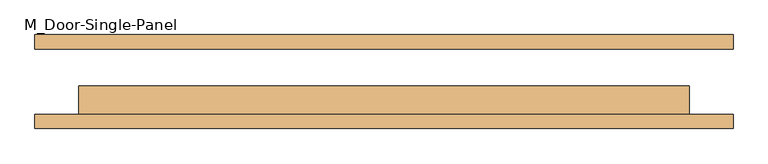
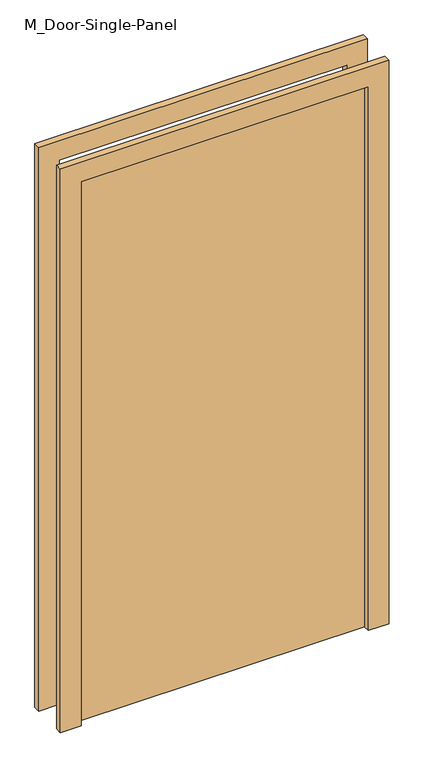
"""IFC4 building model written with IfcOpenShell, lengths in millimetres: door geometry, M_Door-Single-Panel."""

from ifc_helpers import new_model, si_unit, frame, origin, origin_with_axes, place, context, project, spatial, polyline, outline, extrude, source, transform, mapped, element, save


def m_door_single_panel_05506f71(model_context):
    return source(origin(), model_context, "Body", "SweptSolid", [
        extrude(outline(polyline([(533.4, -7.15), (533.4, -57.15), (-533.4, -57.15), (-533.4, -7.15), (533.4, -7.15)])), origin_with_axes(), (0.0, 0.0, 1.0), 2133.6),
        extrude(outline(polyline([(2209.8, 609.6), (2209.8, -609.6), (0.0, -609.6), (0.0, -533.4), (2133.6, -533.4), (2133.6, 533.4), (0.0, 533.4), (0.0, 609.6), (2209.8, 609.6)])), frame((0.0, 57.15, 0.0), z_axis=(0.0, 1.0, 0.0), x_axis=(0.0, 0.0, 1.0)), (0.0, 0.0, 1.0), 25.0),
        extrude(outline(polyline([(2209.8, -609.6), (0.0, -609.6), (0.0, -533.4), (2133.6, -533.4), (2133.6, 533.4), (0.0, 533.4), (0.0, 609.6), (2209.8, 609.6), (2209.8, -609.6)])), frame((0.0, -82.15, 0.0), z_axis=(0.0, 1.0, 0.0), x_axis=(0.0, 0.0, 1.0)), (0.0, 0.0, 1.0), 25.0),
    ])


if __name__ == "__main__":
    model = new_model("IFC4")
    model_context = context("Model", 3, world=origin())
    ifc_project = project(units=[si_unit("LENGTHUNIT", "METRE", prefix="MILLI")], contexts=[model_context])
    site = spatial("IfcSite", under=ifc_project)
    building = spatial("IfcBuilding", under=site)
    placement = place(None, origin())
    m_door_single_panel_shape = m_door_single_panel_05506f71(model_context)
    element("IfcDoor", 1, ObjectType="M_Door-Single-Panel", at=placement, inside=building, context=model_context, shape_type="MappedRepresentation", body=[
        mapped(m_door_single_panel_shape, transform((0.0, 0.0, 0.0), x_axis=(1.0, 0.0, 0.0), y_axis=(0.0, 1.0, 0.0), z_axis=(0.0, 0.0, 1.0))),
    ])
    save(model, "model.ifc")

# Revit data of these elements
# Type "M_Door-Single-Panel"
#   Type Mark = "14"
#   Construction Type Id = "DOOR"
#   Assembly Code = "C1020300"
#   Analytic Construction = "Wooden"
#   Thickness = 0' - 1.9685"
#   Thermal Resistance (R) = 2.5876 (h·ft²·°F)/BTU
#   Swing Angle [instance default] = 90.00°
#   Heat Transfer Coefficient (U) = 0.3865 BTU/(h·ft²·°F)
#   Height = 7' - 0"
#   Trim Projection Ext = 0' - 0.98425"
#   Trim Projection Int = 0' - 0.98425"
#   Trim Width = 0' - 3.14961"
#   Width = 3' - 6"
#   Define Thermal Properties by = 1
#   Panel Material = Wood - Birch - Solid Stained Light Low Gloss
#   Trim Material = Paint - Sienna
#   Visual Light Transmittance = 0
#   Solar Heat Gain Coefficient = 0
#   Function = (empty or 0)
#   Wall Closure = (empty or 0)
# Element 1 (IfcDoor, "M_Door-Single-Panel")
#   Materials on its faces: "Paint - Sienna", "Wood - Birch - Solid Stained Light Low Gloss"
# Materials
#   "Wood - Birch - Solid Stained Light Low Gloss": class "Wood", colour RGB 210 159 95, transparency 0, Cost = 0
#   "Paint - Sienna": colour RGB 118 70 51, transparency 0, Cost = 0
